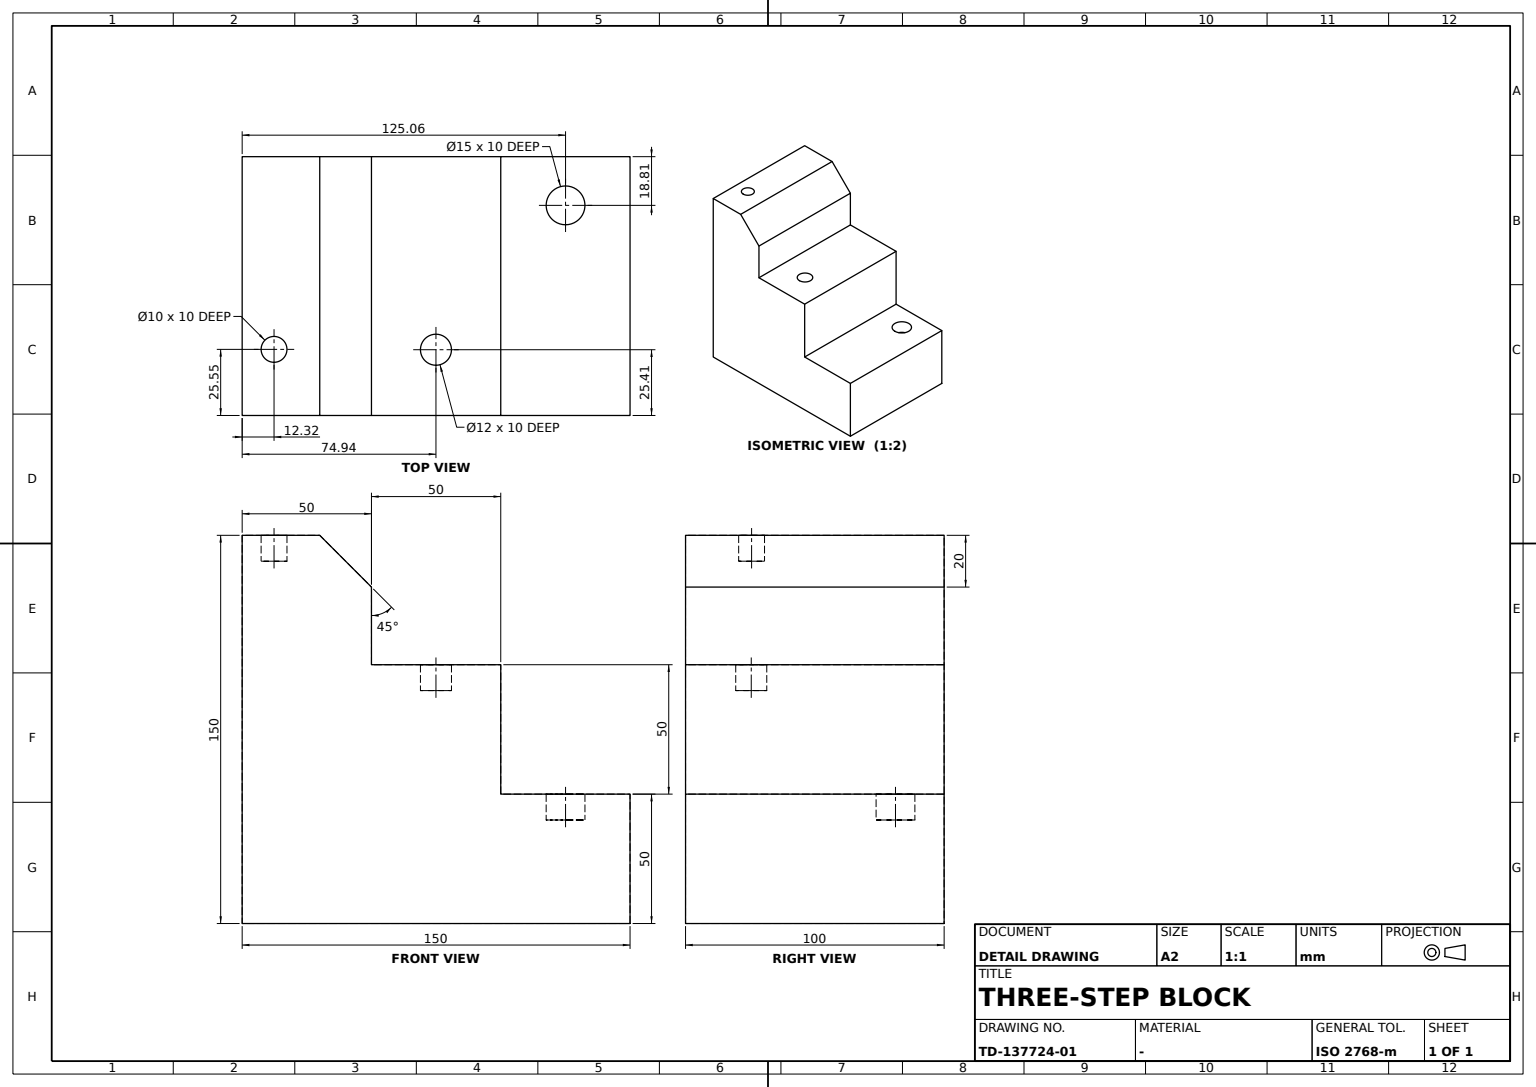
CATIA V5 part; units mm, degrees
sketch "Sketch1" plane through (0, 0, 0) normal (1, 0, 0) x (0, 1, 0)
  point P0 (-75, 75)
  line L0 (-75, 75) -> (-75, -75)
  point P1 (-75, -75)
  line L1 (-75, -75) -> (75, -75)
  line L2 (75, -75) -> (75, -25)
  line L3 (75, -25) -> (25, -25)
  line L4 (25, -25) -> (25, 25)
  line L5 (25, 25) -> (-25, 25)
  line L6 (-25, 25) -> (-25, 75)
  line L7 (-25, 75) -> (-75, 75)
  dimension "length L1" = 150
  dimension "length L0" = 150
  dimension "length L2" = 50
  dimension "length L4" = 50
  dimension "length L7" = 50
  dimension "length L5" = 50
  constraint vertical L0 y-axis
  constraint vertical L2 y-axis
  constraint vertical L4 y-axis
  constraint vertical L6 y-axis
  constraint horizontal L1 x-axis
  constraint horizontal L3 x-axis
  constraint horizontal L5 x-axis
  constraint horizontal L7 x-axis
  constraint symmetry P0 P1 x-axis
  constraint symmetry L0 L2 y-axis
extrude "Pad1" add sketch "Sketch1" along normal mid plane 100
chamfer "Chamfer1" distance 20 angle 45 1 edges at (0, -25, 75)
sketch "Sketch2" plane through (24.4545, -62.6752, 75) normal (0, 0, 1) x (1, 0, 0)
  point P0 (0, 0)
hole "Hole1" at (24.4545, -62.6752, 75) direction (0, 0, -1) diameter 10 depth 10
sketch "Sketch3" plane through (24.5909, -0.0597, 25) normal (0, 0, 1) x (1, 0, 0)
  point P0 (0, 0)
hole "Hole2" at (24.5909, -0.0597, 25) direction (0, 0, -1) diameter 12 depth 10
sketch "Sketch4" plane through (-31.1874, 50.0594, -25) normal (0, 0, 1) x (1, 0, 0)
  point P0 (0, 0)
hole "Hole3" at (-31.1874, 50.0594, -25) direction (0, 0, -1) diameter 15 depth 10
